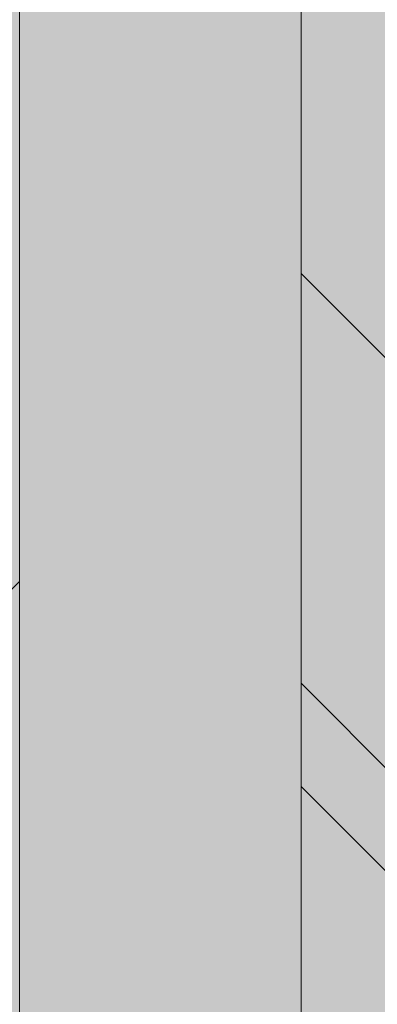
# Model space of a CAD drawing. Units: inches. Extents: x 844 to 2234, y 346 to 1084.
# Tile 78 of 93: x 1998.757 to 1999.568, y 706.514 to 708.742. Entities that reach past the tile are written whole.
import ezdxf

# ---------------------------------------------------------------- set-up
doc = ezdxf.new("R2010")
doc.units = ezdxf.units.IN
doc.header["$MEASUREMENT"] = 0
for name, color, linetype, lineweight in [('A-ANNO-DIMS', 2, 'Continuous', 18), ('furniture', 8, 'Continuous', 18), ('RA-AP-01$0$INT', 35, 'Continuous', 5)]:
    doc.layers.add(name, color=color, linetype=linetype, lineweight=lineweight)
doc.layers.add('RA-AP-01$0$FURN', color=3, linetype='Continuous')
doc.layers.add('RA-AP-01$0$WOOD', color=64, linetype='Continuous')
doc.styles.get("Standard").update_dxf_attribs({"font": 'arial.ttf'})
doc.dimstyles.get("Standard").update_dxf_attribs({"dimtxt": 6, "dimasz": 3, "dimexe": 0.18, "dimexo": 0.0625, "dimgap": 0.09, "dimtad": 0, "dimtih": 1, "dimtoh": 1, "dimdec": 1, "dimzin": 0, "dimdsep": 46, "dimlunit": 3, "dimtxsty": 'Standard', "dimblk": 'ARCHTICK', "dimcen": 0.09, "dimadec": 0, "dimazin": 0, "dimtfac": 1, "dimtdec": 1, "dimtofl": 0, "dimtmove": 0, "dimatfit": 3, "dimfxl": 1, "dimtolj": 1, "dimtzin": 0, "dimarcsym": 0})

# ---------------------------------------------------------------- blocks, each defined once
blk = doc.blocks.new('A$C18D01794')
at = {"layer": 'RA-AP-01$0$INT'}
h = blk.add_hatch(color=256, dxfattribs=at)
h.paths.add_polyline_path([(4.505206456958071, -7.585498806127123), (4.46934859260189, -7.549640941759413), (4.505206456958071, -7.513783077414768), (4.505206456958071, -7.381963272220687), (4.469348592616735, -7.346105407867824), (4.505206456958071, -7.310247543514964), (4.505206456958071, -7.178427738324996), (4.469348592586679, -7.142569873965138), (4.505206456952245, -7.106712009588038), (4.476922185709333, -7.106712009588038), (4.455206456960671, -7.128427738343681), (4.433490728198047, -7.106712009588038), (4.405206456946033, -7.106712009588036), (4.441064321339216, -7.142569873969684), (4.40520645695807, -7.178427738362358), (4.405206456958072, -7.310247543472698), (4.441064321364728, -7.346105407867826), (4.40520645695807, -7.381963272262947), (4.40520645695807, -7.513783077378263), (4.441064321354429, -7.549640941786153), (4.405206456958072, -7.585498806170974), (4.405206456958072, -7.717318611286652), (4.441064321333084, -7.753176475673194), (4.405206456958072, -7.789034340036673), (4.405206456958072, -8.006712009588039), (4.644348592588106, -8.006712009588039), (4.680206456964639, -7.970854145211967), (4.716064321341165, -8.006712009588039), (4.869348592586113, -8.006712009588039), (4.905206456964143, -7.970854145210465), (4.941064321342174, -8.006712009588039), (5.094348592587118, -8.006712009588037), (5.130206456963649, -7.970854145211967), (5.166064321340178, -8.006712009588039), (5.405206456958072, -8.006712009588039), (5.405206456958072, -7.789034340024526), (5.369348592595202, -7.753176475673196), (5.40520645695807, -7.717318611298797), (5.40520645695807, -7.585498806158829), (5.369348592573859, -7.549640941786151), (5.40520645695807, -7.51378307739041), (5.40520645695807, -7.381963272250803), (5.36934859256356, -7.346105407867824), (5.405206456958072, -7.310247543484846), (5.405206456958072, -7.178427738350217), (5.369348592589068, -7.142569873969682), (5.405206456982249, -7.106712009588038), (5.376922185730244, -7.106712009588038), (5.355206456967613, -7.128427738343679), (5.333490728218955, -7.10671200958804), (5.305206456976043, -7.106712009588042), (5.341064321341609, -7.142569873965136), (5.305206456958072, -7.178427738337141), (5.305206456958072, -7.310247543502816), (5.34106432131155, -7.346105407867824), (5.305206456958072, -7.381963272232832), (5.30520645695807, -7.513783077402624), (5.341064321326395, -7.549640941759413), (5.305206456958072, -7.585498806139263), (5.305206456958072, -7.717318611299605), (5.341064321347738, -7.753176475677737), (5.305206456958072, -7.78903434007894), (5.30520645695807, -7.906712009588039), (5.166064321336834, -7.906712009588039), (5.130206456963647, -7.942569873961684), (5.094348592590464, -7.906712009588039), (4.941064321338827, -7.906712009588041), (4.905206456964145, -7.942569873963183), (4.869348592589459, -7.906712009588039), (4.716064321337822, -7.906712009588041), (4.680206456964641, -7.942569873961684), (4.644348592591453, -7.906712009588039), (4.505206456958071, -7.906712009588039), (4.505206456958071, -7.789034340066795), (4.469348592580545, -7.753176475677738), (4.505206456958071, -7.717318611311748)])
h.paths.add_polyline_path([(4.485206456974132, -7.709034340046354), (4.45520645695909, -7.739034340051736), (4.425206456974128, -7.709034340057131), (4.425206456993394, -7.593783077384998), (4.45520645699153, -7.563783077396511), (4.485206456993396, -7.593783077408017)], flags=16)
h.paths.add_polyline_path([(4.455206456954537, -7.767318611299197), (4.485206456958242, -7.797318611312542), (4.48520645695951, -7.912569873958716), (4.45520645695415, -7.942569873954422), (4.425206456957888, -7.912569873967813), (4.425206456957888, -7.797318611286197)], flags=16)
h.paths.add_polyline_path([(4.455206456964794, -7.535498806149051), (4.42520645696469, -7.5054988061393), (4.425206456983954, -7.390247543486406), (4.455206456990734, -7.360247543489279), (4.485206456983953, -7.39024754349214), (4.485206456964687, -7.505498806158811)], flags=16)
h.paths.add_polyline_path([(4.499348592588947, -7.926712009585049), (4.636064321340932, -7.926712009585049), (4.666064321342317, -7.956712009586821), (4.636064321343707, -7.986712009585048), (4.499348592575121, -7.986712009585048), (4.469348592591685, -7.956712009591957)], flags=16)
h.paths.add_polyline_path([(4.425206456957888, -7.940854145195974), (4.471064321332215, -7.986712009585049), (4.425206456957888, -7.986712009585049)], flags=16)
h.paths.add_polyline_path([(4.455206456990734, -7.331963272246367), (4.425206456989053, -7.301963272254337), (4.425206456969784, -7.186712009596224), (4.455206456965226, -7.156712009591144), (4.485206456969787, -7.186712009586051), (4.485206456989053, -7.301963272238404)], flags=16)
h.paths.add_polyline_path([(4.72434859258714, -7.926712009586255), (4.861064321340141, -7.926712009586248), (4.891064321340324, -7.956712009586823), (4.861064321340513, -7.986712009586252), (4.724348592586768, -7.986712009586252), (4.694348592586956, -7.956712009586821)], flags=16)
h.paths.add_polyline_path([(4.919348592587961, -7.956712009586821), (4.949348592588145, -7.92671200958625), (5.08606432134115, -7.926712009586253), (5.116064321341327, -7.956712009586823), (5.086064321341519, -7.986712009586252), (4.949348592587774, -7.986712009586252)], flags=16)
h.paths.add_polyline_path([(5.144348592585967, -7.956712009586823), (5.174348592587358, -7.926712009585049), (5.311064321339338, -7.926712009585049), (5.3410643213366, -7.956712009591957), (5.311064321353163, -7.986712009585048), (5.174348592584576, -7.986712009585048)], flags=16)
h.paths.add_polyline_path([(5.32520645693489, -7.593783077408021), (5.355206456936755, -7.563783077396511), (5.385206456934894, -7.593783077384998), (5.38520645695416, -7.709034340057128), (5.355206456969194, -7.739034340051736), (5.325206456954153, -7.709034340046352)], flags=16)
h.paths.add_polyline_path([(5.325206456970042, -7.797318611312542), (5.355206456973747, -7.767318611299197), (5.385206456970398, -7.7973186112862), (5.385206456970398, -7.912569873967816), (5.355206456974136, -7.942569873954422), (5.325206456968778, -7.912569873958716)], flags=16)
h.paths.add_polyline_path([(5.325206456963599, -7.505498806158811), (5.325206456944333, -7.39024754349214), (5.355206456937552, -7.360247543489279), (5.385206456944332, -7.39024754348641), (5.385206456963596, -7.505498806139303), (5.355206456963492, -7.53549880614905)], flags=16)
h.paths.add_polyline_path([(5.32520645693923, -7.301963272238403), (5.3252064569585, -7.186712009586051), (5.355206456963062, -7.156712009591142), (5.3852064569585, -7.186712009596224), (5.385206456939234, -7.301963272254338), (5.355206456937552, -7.331963272246369)], flags=16)
h.paths.add_polyline_path([(5.339348592596071, -7.986712009585048), (5.385206456970398, -7.940854145195972), (5.385206456970396, -7.986712009585048)], flags=16)
h = blk.add_hatch(color=256, dxfattribs=at)
h.paths.add_polyline_path([(4.469348592586677, -7.142569873965136), (4.505206456958073, -7.178427738324996), (4.505206456958071, -7.106712009582215)])
h.paths.add_polyline_path([(4.455206456960671, -7.128427738343681), (4.476922185709333, -7.106712009588038), (4.433490728198045, -7.106712009588038)])
h.paths.add_polyline_path([(4.405206456958073, -7.178427738362358), (4.441064321339218, -7.142569873969684), (4.40520645695807, -7.106712009600073)])
h.paths.add_polyline_path([(4.425206456989053, -7.301963272254335), (4.455206456990736, -7.331963272246371), (4.485206456989055, -7.301963272238399), (4.48520645696979, -7.186712009586054), (4.455206456965227, -7.15671200959114), (4.425206456969784, -7.186712009596224)])
h.paths.add_polyline_path([(4.505206456958073, -7.381963272220689), (4.505206456958071, -7.310247543514961), (4.469348592616738, -7.346105407867826)])
h.paths.add_polyline_path([(4.425206456964688, -7.5054988061393), (4.455206456964794, -7.535498806149051), (4.485206456964689, -7.505498806158811), (4.485206456983951, -7.390247543492138), (4.455206456990736, -7.360247543489277), (4.425206456983956, -7.39024754348641)])
h.paths.add_polyline_path([(4.425206456974126, -7.709034340057128), (4.455206456959092, -7.739034340051736), (4.485206456974132, -7.709034340046356), (4.485206456993396, -7.593783077408017), (4.45520645699153, -7.563783077396511), (4.425206456993394, -7.593783077384999)])
h.paths.add_polyline_path([(4.46934859260189, -7.549640941759415), (4.505206456958071, -7.585498806127123), (4.505206456958073, -7.513783077414766)])
h.paths.add_polyline_path([(4.405206456958073, -7.585498806170972), (4.441064321354427, -7.549640941786151), (4.405206456958072, -7.513783077378263)])
h.paths.add_polyline_path([(4.405206456958072, -7.789034340036673), (4.441064321333084, -7.753176475673194), (4.405206456958072, -7.71731861128665)])
h.paths.add_polyline_path([(4.469348592580547, -7.75317647567774), (4.505206456958071, -7.789034340066795), (4.505206456958071, -7.717318611311744)])
h.paths.add_polyline_path([(4.425206456957888, -7.912569873967814), (4.45520645695415, -7.942569873954422), (4.485206456959507, -7.912569873958718), (4.48520645695824, -7.797318611312542), (4.455206456954537, -7.767318611299197), (4.425206456957888, -7.797318611286202)])
h.paths.add_polyline_path([(4.425206456957888, -7.986712009585049), (4.471064321332215, -7.986712009585049), (4.425206456957888, -7.940854145195972)])
h.paths.add_polyline_path([(4.499348592575121, -7.986712009585048), (4.636064321343707, -7.986712009585049), (4.666064321342317, -7.956712009586823), (4.636064321340932, -7.926712009585049), (4.499348592588945, -7.926712009585049), (4.469348592591685, -7.95671200959196)])
h.paths.add_polyline_path([(4.680206456964641, -7.942569873961684), (4.716064321337824, -7.906712009588039), (4.644348592591454, -7.906712009588039)])
h.paths.add_polyline_path([(4.644348592588108, -8.006712009588039), (4.716064321341167, -8.006712009588039), (4.680206456964637, -7.970854145211964)])
h.paths.add_polyline_path([(4.724348592586768, -7.98671200958625), (4.861064321340514, -7.986712009586252), (4.891064321340324, -7.956712009586819), (4.861064321340141, -7.92671200958625), (4.724348592587134, -7.926712009586255), (4.694348592586957, -7.956712009586821)])
h.paths.add_polyline_path([(4.905206456964143, -7.942569873963183), (4.941064321338827, -7.906712009588039), (4.869348592589457, -7.906712009588037)])
h.paths.add_polyline_path([(4.869348592586113, -8.006712009588039), (4.941064321342172, -8.006712009588037), (4.905206456964145, -7.970854145210463)])
h.paths.add_polyline_path([(4.949348592587774, -7.986712009586252), (5.086064321341521, -7.986712009586252), (5.116064321341329, -7.956712009586823), (5.08606432134115, -7.926712009586253), (4.949348592588145, -7.92671200958625), (4.919348592587961, -7.956712009586819)])
h.paths.add_polyline_path([(5.130206456963645, -7.942569873961684), (5.166064321336834, -7.906712009588039), (5.094348592590464, -7.906712009588039)])
h.paths.add_polyline_path([(5.094348592587119, -8.006712009588039), (5.166064321340178, -8.006712009588039), (5.130206456963651, -7.970854145211967)])
h.paths.add_polyline_path([(5.174348592584578, -7.986712009585048), (5.311064321353163, -7.986712009585048), (5.341064321336602, -7.956712009591958), (5.31106432133934, -7.926712009585049), (5.174348592587352, -7.926712009585049), (5.144348592585969, -7.956712009586823)])
h.paths.add_polyline_path([(5.325206456968778, -7.912569873958718), (5.355206456974136, -7.942569873954422), (5.385206456970396, -7.912569873967814), (5.385206456970396, -7.797318611286199), (5.355206456973747, -7.767318611299197), (5.325206456970044, -7.797318611312544)])
h.paths.add_polyline_path([(5.339348592596073, -7.986712009585048), (5.385206456970396, -7.986712009585049), (5.385206456970398, -7.94085414519597)])
h.paths.add_polyline_path([(5.325206456954155, -7.709034340046354), (5.355206456969194, -7.739034340051734), (5.38520645695416, -7.709034340057128), (5.385206456934896, -7.593783077384999), (5.355206456936758, -7.563783077396513), (5.325206456934888, -7.593783077408019)])
h.paths.add_polyline_path([(5.305206456958072, -7.789034340078938), (5.341064321347739, -7.753176475677738), (5.305206456958072, -7.717318611299605)])
h.paths.add_polyline_path([(5.369348592595204, -7.753176475673194), (5.40520645695807, -7.789034340024526), (5.405206456958072, -7.717318611298798)])
h.paths.add_polyline_path([(5.405206456958072, -7.585498806158831), (5.405206456958072, -7.513783077390407), (5.369348592573857, -7.549640941786151)])
h.paths.add_polyline_path([(5.305206456958072, -7.585498806139266), (5.341064321326393, -7.549640941759413), (5.305206456958072, -7.513783077402626)])
h.paths.add_polyline_path([(5.325206456963599, -7.50549880615881), (5.355206456963494, -7.535498806149055), (5.385206456963598, -7.505498806139302), (5.385206456944334, -7.390247543486411), (5.355206456937552, -7.360247543489279), (5.325206456944333, -7.39024754349214)])
h.paths.add_polyline_path([(5.305206456958072, -7.38196327223283), (5.341064321311551, -7.346105407867824), (5.305206456958072, -7.31024754350282)])
h.paths.add_polyline_path([(5.325206456939231, -7.301963272238404), (5.355206456937552, -7.331963272246369), (5.385206456939235, -7.301963272254335), (5.385206456958502, -7.186712009596224), (5.355206456963061, -7.156712009591142), (5.3252064569585, -7.186712009586051)])
h.paths.add_polyline_path([(5.404581768715993, -7.381338584008926, -0.001217816984214), (5.405206456958072, -7.381112009582329), (5.405206456958072, -7.310247543484846), (5.369348592563558, -7.346105407867826)])
h.paths.add_polyline_path([(5.36934859258907, -7.142569873969684), (5.40520645695807, -7.178427738350215), (5.405206456958072, -7.106712009612218)])
h.paths.add_polyline_path([(5.355206456967613, -7.128427738343683), (5.376922185730239, -7.106712009588038), (5.333490728218953, -7.10671200958804)])
h.paths.add_polyline_path([(5.30520645695807, -7.178427738337139), (5.341064321341609, -7.142569873965134), (5.305206456958074, -7.10671200957007)])
blk.add_hatch(color=256, dxfattribs=at).paths.add_polyline_path([(4.505206456958071, -7.906712009588039), (5.305206456958072, -7.906712009588039), (5.305206456958072, -7.106712009588038), (5.255206456951893, -7.106712009588036), (5.25520645694868, -7.856712009570104), (4.555206456959269, -7.856712009588616), (4.555206456956052, -7.106712009588038), (4.505206456958073, -7.106712009588038)])
h = blk.add_hatch(color=256, dxfattribs=at)
h.paths.add_polyline_path([(4.585917135068448, -7.856712009587804), (4.614201406330596, -7.856712009587056), (4.668846067270487, -7.802067348644738), (4.723490728212344, -7.856712009584164), (4.771774999457151, -7.856712009582887), (4.826419660396886, -7.80206734864072), (4.862780050090322, -7.838427738332541), (4.844495778842715, -7.856712009580965), (4.862780050090411, -7.856712009580482), (4.905206456960182, -7.814285602707865), (4.947632863832445, -7.856712009578238), (4.965917135079675, -7.856712009577755), (4.947632863831759, -7.838427738330656), (4.983993253523576, -7.802067348637219), (5.038637914464627, -7.856712009575829), (5.08692218571208, -7.856712009574554), (5.141566846649976, -7.802067348634224), (5.196211507589851, -7.856712009571666), (5.224495778822615, -7.856712009570916), (4.905206456953975, -7.537422687702283)])
h.paths.add_polyline_path([(4.895206456956031, -7.575706958950402), (4.895206456958921, -7.684996280828174), (4.840561796018589, -7.630351619890275)], flags=16)
h.paths.add_polyline_path([(4.915206456955638, -7.575706958949956), (4.969851117895509, -7.630351619887399), (4.915206456957609, -7.684996280827732)], flags=16)
h.paths.add_polyline_path([(4.826419660395175, -7.644493755514321), (4.881064321335613, -7.699138416452331), (4.771774999456703, -7.69913841645522)], flags=16)
h.paths.add_polyline_path([(4.983993253519558, -7.644493755510815), (5.038637914460456, -7.699138416449285), (4.929348592581548, -7.69913841645126)], flags=16)
h.paths.add_polyline_path([(4.881064321336025, -7.719138416452334), (4.826419660397532, -7.773783077393256), (4.771774999457062, -7.719138416455217)], flags=16)
h.paths.add_polyline_path([(4.929348592582019, -7.71913841645126), (5.038637914460982, -7.719138416449284), (4.983993253522945, -7.773783077389749)], flags=16)
h.paths.add_polyline_path([(4.895206456960191, -7.733280552075633), (4.895206456962115, -7.806001331460164), (4.876922185715016, -7.824285602708492), (4.840561796021581, -7.787925213016675)], flags=16)
h.paths.add_polyline_path([(4.915206456958487, -7.733280552075187), (4.969851117899527, -7.787925213013798), (4.933490728206909, -7.824285602708034), (4.9152064569598, -7.806001331461736)], flags=16)
h.paths.add_polyline_path([(4.757632863832376, -7.733280552079264), (4.812277524772842, -7.787925213017304), (4.757632863834348, -7.842569873958233)], flags=16)
h.paths.add_polyline_path([(4.737632863832376, -7.73328055207979), (4.737632863834348, -7.842569873958701), (4.682988202893906, -7.787925213020692)], flags=16)
h.paths.add_polyline_path([(5.05278005008503, -7.733280552072701), (5.052780050087917, -7.842569873951664), (4.998135389146995, -7.787925213013169)], flags=16)
h.paths.add_polyline_path([(5.072780050085024, -7.733280552072333), (5.127424711025931, -7.787925213010806), (5.072780050087916, -7.842569873951244)], flags=16)
h.paths.add_polyline_path([(4.935917135072783, -7.506712009583784), (5.255206456948811, -7.826001331459767), (5.255206456948932, -7.797717060211899), (5.200561796010279, -7.743072399273238), (5.255206456949403, -7.688427738334128), (5.25520645694961, -7.640143467086677), (5.200561796009787, -7.585498806146837), (5.236922185702417, -7.549138416454212), (5.255206456949919, -7.56742268770172), (5.255206456949998, -7.549138416454178), (5.212780050078687, -7.506712009583814), (5.25520645695036, -7.464285602712145), (5.255206456950438, -7.446001331464763), (5.236922185702424, -7.464285602712779), (5.200561796009796, -7.427925213020149), (5.255206456950753, -7.373280552079203), (5.25520645695096, -7.324996280834394), (5.200561796010322, -7.270351619893748), (5.255206456951428, -7.215706958952649), (5.255206456951547, -7.187422687705071)])
h.paths.add_polyline_path([(5.042988202883395, -7.42792521302065), (5.097632863823085, -7.373280552080975), (5.097632863822622, -7.482569873959883)], flags=16)
h.paths.add_polyline_path([(5.028846067259663, -7.442067348644384), (5.083490728198774, -7.496712009583504), (4.974201406321001, -7.496712009583035)], flags=16)
h.paths.add_polyline_path([(5.117632863823087, -7.37328055208089), (5.172277524762331, -7.42792521302015), (5.11763286382262, -7.482569873959851)], flags=16)
h.paths.add_polyline_path([(5.08349072819877, -7.516712009582191), (5.028846067259652, -7.571356670521302), (4.974201406320998, -7.516712009582638)], flags=16)
h.paths.add_polyline_path([(5.131774999446817, -7.35913841645716), (5.186419660386065, -7.413783077396415), (5.241064321325782, -7.359138416456712)], flags=17)
h.paths.add_polyline_path([(5.131774999446228, -7.496712009583703), (5.186419660386065, -7.442067348643883), (5.222780050079488, -7.478427738337313), (5.204495778832781, -7.496712009584014)], flags=16)
h.paths.add_polyline_path([(5.097632863822613, -7.530854145205813), (5.097632863823061, -7.640143467084723), (5.042988202883383, -7.585498806145032)], flags=16)
h.paths.add_polyline_path([(5.131774999446899, -7.339138416457162), (5.241064321325809, -7.339138416456712), (5.186419660386591, -7.284493755517479)], flags=17)
h.paths.add_polyline_path([(5.131774999446226, -7.516712009581999), (5.204495778830767, -7.516712009581702), (5.22278005007868, -7.534996280829206), (5.186419660386049, -7.571356670521828)], flags=16)
h.paths.add_polyline_path([(5.11763286382262, -7.530854145205852), (5.17227752476232, -7.585498806145562), (5.117632863823064, -7.64014346708481)], flags=16)
h.paths.add_polyline_path([(5.186419660386069, -7.599640941770585), (5.241064321325754, -7.654285602710281), (5.131774999446791, -7.654285602709814)], flags=16)
h.paths.add_polyline_path([(5.131774999446872, -7.674285602709813), (5.24106432132578, -7.674285602710282), (5.186419660386554, -7.728930263649504)], flags=16)
h.paths.add_polyline_path([(5.255206456951811, -7.126001331467467), (5.255206456951895, -7.106712009588038), (4.555206456956052, -7.106712009588038), (4.555206456956136, -7.12600133146746), (4.905206456953973, -7.476001331465289)])
h.paths.add_polyline_path([(4.983993253513404, -7.368930263651977), (4.92934859257295, -7.314285602713969), (5.03863791445186, -7.314285602711063)], flags=16)
h.paths.add_polyline_path([(4.969851117889988, -7.383072399276016), (4.915206456952556, -7.437717060215906), (4.915206456949648, -7.328427738338133)], flags=16)
h.paths.add_polyline_path([(4.929348592572535, -7.294285602713971), (4.983993253511019, -7.239640941773039), (5.038637914451496, -7.294285602711065)], flags=16)
h.paths.add_polyline_path([(5.052780050074912, -7.280143467087016), (4.998135389134438, -7.225498806148989), (5.052780050072919, -7.170854145208052)], flags=16)
h.paths.add_polyline_path([(5.07278005007491, -7.280143467086489), (5.072780050072918, -7.170854145207579), (5.127424711013374, -7.225498806145578)], flags=16)
h.paths.add_polyline_path([(4.89520645695295, -7.437717060216355), (4.840561796013067, -7.383072399278919), (4.895206456950961, -7.328427738338582)], flags=16)
h.paths.add_polyline_path([(4.915206456948365, -7.280143467090674), (4.915206456946434, -7.207422687704125), (4.933490728192729, -7.18913841645701), (4.969851117886972, -7.225498806149623)], flags=16)
h.paths.add_polyline_path([(4.881064321327021, -7.314285602715054), (4.82641966038902, -7.368930263655506), (4.771774999448108, -7.314285602717047)], flags=16)
h.paths.add_polyline_path([(4.895206456950073, -7.280143467091125), (4.840561796009022, -7.225498806152518), (4.876922185700835, -7.18913841645908), (4.895206456948749, -7.207422687706589)], flags=16)
h.paths.add_polyline_path([(4.983993253510392, -7.211356670525576), (4.947632863816944, -7.174996280833758), (4.965917135064043, -7.156712009585847), (5.038637914448995, -7.156712009584522)], flags=16)
h.paths.add_polyline_path([(4.881064321326543, -7.294285602715056), (4.771774999447578, -7.294285602717046), (4.826419660385607, -7.239640941776569)], flags=16)
h.paths.add_polyline_path([(4.905206456946447, -7.19913841645844), (4.862780050074785, -7.156712009587725), (4.947632863816685, -7.156712009586302)], flags=16)
h.paths.add_polyline_path([(5.14156684663679, -7.211356670521528), (5.086922185696452, -7.156712009583639), (5.196211507574223, -7.156712009581651)], flags=16)
h.paths.add_polyline_path([(4.8264196603837, -7.211356670529104), (4.771774999442643, -7.156712009590501), (4.8444957788276, -7.156712009588568), (4.862780050075511, -7.17499628083566)], flags=16)
h.paths.add_polyline_path([(4.812277524760289, -7.225498806153156), (4.757632863822258, -7.28014346709363), (4.757632863819352, -7.170854145214669)], flags=16)
h.paths.add_polyline_path([(4.73763286382226, -7.280143467093997), (4.682988202881349, -7.22549880615554), (4.737632863819352, -7.170854145215086)], flags=16)
h.paths.add_polyline_path([(4.723490728195188, -7.156712009591787), (4.668846067257299, -7.211356670532127), (4.614201406317417, -7.156712009594693)], flags=16)
h.paths.add_polyline_path([(4.597632863829262, -7.506712009583814), (4.555206456957951, -7.54913841645418), (4.555206456958029, -7.56742268770172), (4.573490728205535, -7.549138416454212), (4.609851117898167, -7.585498806146839), (4.555206456958338, -7.640143467086675), (4.555206456958546, -7.688427738334125), (4.60985111789767, -7.743072399273238), (4.555206456959015, -7.797717060211899), (4.555206456959138, -7.826001331459767), (4.874495778835167, -7.506712009583786), (4.5552064569564, -7.187422687705062), (4.555206456956523, -7.215706958952644), (4.609851117897629, -7.270351619893746), (4.555206456956988, -7.324996280834396), (4.555206456957198, -7.373280552079195), (4.609851117898153, -7.427925213020147), (4.573490728205528, -7.464285602712779), (4.555206456957507, -7.446001331464756), (4.555206456957585, -7.464285602712143)])
h.paths.add_polyline_path([(4.712780050085332, -7.482569873959882), (4.712780050084863, -7.373280552080972), (4.767424711024555, -7.42792521302065)], flags=16)
h.paths.add_polyline_path([(4.726922185709173, -7.496712009583504), (4.781566846648288, -7.442067348644384), (4.836211507586949, -7.496712009583033)], flags=16)
h.paths.add_polyline_path([(4.692780050085327, -7.482569873959851), (4.638135389145619, -7.427925213020149), (4.692780050084865, -7.373280552080892)], flags=16)
h.paths.add_polyline_path([(4.726922185709182, -7.516712009582191), (4.836211507586949, -7.51671200958264), (4.7815668466483, -7.571356670521304)], flags=16)
h.paths.add_polyline_path([(4.678637914461726, -7.496712009583706), (4.605917135075169, -7.496712009584014), (4.587632863828464, -7.478427738337311), (4.623993253521887, -7.442067348643881)], flags=16)
h.paths.add_polyline_path([(4.712780050085336, -7.530854145205816), (4.767424711024568, -7.585498806145034), (4.71278005008489, -7.640143467084724)], flags=16)
h.paths.add_polyline_path([(4.678637914461726, -7.516712009582001), (4.623993253521899, -7.571356670521829), (4.587632863829271, -7.534996280829206), (4.605917135077185, -7.5167120095817)], flags=16)
h.paths.add_polyline_path([(4.692780050085336, -7.530854145205848), (4.692780050084889, -7.64014346708481), (4.638135389145632, -7.585498806145562)], flags=16)
h.paths.add_polyline_path([(4.623993253521885, -7.413783077396415), (4.678637914461131, -7.359138416457161), (4.56934859258217, -7.359138416456712)], flags=17)
h.paths.add_polyline_path([(4.623993253521901, -7.599640941770568), (4.678637914461158, -7.654285602709814), (4.569348592582195, -7.654285602710281)], flags=16)
h.paths.add_polyline_path([(4.678637914461051, -7.339138416457162), (4.623993253521361, -7.284493755517479), (4.569348592582143, -7.339138416456712)], flags=17)
h.paths.add_polyline_path([(4.678637914461076, -7.674285602709813), (4.623993253521399, -7.728930263649504), (4.569348592582167, -7.674285602710281)], flags=16)
h = blk.add_hatch(color=256, dxfattribs=at)
h.paths.add_polyline_path([(5.028846067259997, -7.571356670520955), (4.974201406321342, -7.516712009582294), (5.083490728199115, -7.516712009581846)])
h.paths.add_polyline_path([(4.974201406321344, -7.496712009582688), (5.028846067260004, -7.442067348644037), (5.083490728199117, -7.496712009583157)])
h.paths.add_polyline_path([(5.042988202883738, -7.427925213020309), (5.097632863823428, -7.373280552080627), (5.097632863822963, -7.482569873959537)])
h.paths.add_polyline_path([(5.117632863822961, -7.482569873959509), (5.117632863823428, -7.373280552080546), (5.172277524762674, -7.427925213019804)])
h.paths.add_polyline_path([(5.131774999446572, -7.496712009583358), (5.186419660386406, -7.442067348643536), (5.222780050079831, -7.478427738336961), (5.204495778833122, -7.496712009583667)])
h.paths.add_polyline_path([(5.236922185702764, -7.464285602712433), (5.200561796010139, -7.427925213019802), (5.255206456949971, -7.373280552079975), (5.255206456950271, -7.446001331464927)])
h.paths.add_polyline_path([(5.186419660386412, -7.41378307739607), (5.131774999447164, -7.359138416456815), (5.241064321326123, -7.359138416456366)])
h.paths.add_polyline_path([(5.131774999447238, -7.339138416456815), (5.186419660386934, -7.284493755517132), (5.241064321326153, -7.339138416456368)])
h.paths.add_polyline_path([(5.200561796010663, -7.270351619893402), (5.255206456949324, -7.215706958954747), (5.255206456949777, -7.324996280832518)])
h.paths.add_polyline_path([(5.21278005007903, -7.50671200958347), (5.255206456950223, -7.464285602712278), (5.255206456950696, -7.549138416454185)])
h.paths.add_polyline_path([(5.13177499944657, -7.516712009581652), (5.204495778831106, -7.516712009581354), (5.222780050079024, -7.534996280828858), (5.186419660386397, -7.571356670521485)])
h.paths.add_polyline_path([(5.117632863823405, -7.640143467084465), (5.117632863822955, -7.530854145205498), (5.172277524762665, -7.585498806145217)])
h.paths.add_polyline_path([(5.042988202883727, -7.585498806144689), (5.097632863822957, -7.530854145205474), (5.097632863823407, -7.64014346708438)])
h.paths.add_polyline_path([(5.131774999447135, -7.654285602709467), (5.186419660386394, -7.599640941770219), (5.241064321326097, -7.654285602709933)])
h.paths.add_polyline_path([(5.200561796010128, -7.585498806146492), (5.236922185702758, -7.549138416453866), (5.255206456950264, -7.567422687701371), (5.255206456949948, -7.640143467086325)])
h.paths.add_polyline_path([(5.186419660386895, -7.728930263649157), (5.131774999447213, -7.674285602709467), (5.241064321326127, -7.674285602709934)])
h.paths.add_polyline_path([(5.200561796010624, -7.743072399272893), (5.255206456949745, -7.688427738333778), (5.255206456949276, -7.797717060211553)])
for p, q in [((5.255206456951895, -7.106712009588038), (5.255206456948681, -7.856712009570104)), ((5.25520645694988, -7.464285602712626), (5.255206456950353, -7.549138416454534)), ((5.212780050078687, -7.506712009583814), (5.255206456950353, -7.549138416454534)), ((5.255206456949919, -7.56742268770172), (5.236922185702415, -7.549138416454212)), ((5.305206456939818, -7.58549880615752), (5.341064321310754, -7.549640941775056)), ((5.255206456949918, -7.56742268770172), (5.255206456949605, -7.640143467086671)), ((5.255206456949605, -7.640143467086671), (5.200561796009783, -7.585498806146837))]:
    blk.add_line(p, q, dxfattribs=at)
blk.add_lwpolyline([(5.305206456958072, -7.106712009588038), (5.305206456958072, -7.906712009588039), (4.505206456958071, -7.906712009588039), (4.505206456958071, -7.106712009588038)], dxfattribs=at)
blk = doc.blocks.new('A$C32926AE1')
at = {"layer": 'RA-AP-01$0$WOOD'}
h = blk.add_hatch(color=256, dxfattribs=at)
h.dxf.hatch_style = 1
h.paths.add_polyline_path([(5.157430609644524, 4.573483066760929, -0.1009492694046607), (5.155401577623758, 4.593365984175333, -0.1842662638101597), (5.172249623284174, 4.638795604568598, 0.2056608120311276), (5.179560981299304, 4.661316324430096, 0.3614336704623542), (5.134352340494423, 4.706524965234944, 0.2056608120311297), (5.111831620632933, 4.699213607219793, -0.1842662638101113), (5.066402000239693, 4.682365561559342, -0.1055311479399994), (5.045656153913092, 4.68467289944697, 0.1567636581983829), (4.763886414745334, 4.684672899446966, -0.1055311479399895), (4.743140568418733, 4.68236556155934, -0.1842662638100833), (4.6977109480255, 4.69921360721979, 0.2056608120302612), (4.675190228164109, 4.706524965234949, 0.3614336704708441), (4.629981587358889, 4.66131632442871, 0.2056608120245944), (4.637292945374126, 4.638795604567974, -0.1842662638101024), (4.654140991034615, 4.59336598417475, -0.1009492694055169), (4.652111959013835, 4.573483066760181, 0.021410119221476), (4.629748025606143, 4.156712009541676, 0.0214101192214795), (4.652111959013809, 3.739940952323101, -0.1009492694059586), (4.654140991034615, 3.720058034908448, -0.1842662638100975), (4.637292945374126, 3.674628414515226, 0.2056608120245705), (4.629981587358889, 3.652107694654492, 0.3614336704708879), (4.675190228164113, 3.606899053848249, 0.2056608120302384), (4.697710948025501, 3.614210411863408, -0.1842662638100995), (4.743140568418738, 3.63105845752386, -0.1055311479402541), (4.763886414745388, 3.628751119636215, 0.1567636581983776), (5.045656153913137, 3.628751119636244, -0.1055311479397538), (5.066402000239692, 3.631058457523857, -0.1842662638101067), (5.111831620632931, 3.614210411863407, 0.2056608120310924), (5.134352340494417, 3.606899053848256, 0.3614336704624001), (5.179560981299307, 3.652107694653103, 0.2056608120311314), (5.172249623284175, 3.6746284145146, -0.1842662638101402), (5.155401577623758, 3.72005803490786, -0.1009492694051366), (5.15743060964455, 3.739940952322354, 0.0214101192215073), (5.179794543052287, 4.156712009541468, 0.0214101192215252)])
h.paths.add_polyline_path([(4.639748609479751, 4.156712009541513, 0.0213537860821624), (4.661970494867118, 3.741887061152232, -0.094075836301374), (4.664143710413708, 3.7196126951003, -0.1824818158568985), (4.644813765429836, 3.668037719127816, 0.2056608120245319), (4.639939526753007, 3.653023905887301, 0.3614336704710246), (4.676106439397173, 3.616856993242342, 0.2056608120302234), (4.691120252638095, 3.621731231919122, -0.1824818158602558), (4.742695228611606, 3.641061176902986, -0.1029891339458722), (4.766991894714349, 3.638256818950944, 0.156709409989566), (5.042550673941472, 3.638256818950105, -0.102989133958497), (5.066847340047078, 3.641061176902949, -0.1824818158594995), (5.118422316020358, 3.621731231919103, 0.2056608120311416), (5.133436129261316, 3.616856993242346, 0.3614336704621468), (5.169603041905217, 3.653023905886178, 0.2056608120310986), (5.164728803228477, 3.668037719127177, -0.1824818158565612), (5.145398858244737, 3.719612695099578, -0.0940758363009313), (5.147572073791232, 3.741887061151398, 0.0213537860822023), (5.169793959178681, 4.156712009541451, 0.0213537860822226), (5.147572073791203, 4.571536957931898, -0.0940758363005034), (5.145398858244737, 4.59381132398362, -0.1824818158565587), (5.164728803228476, 4.645386299956021, 0.2056608120311045), (5.169603041905216, 4.66040011319702, 0.3614336704621845), (5.133436129261313, 4.696567025840856, 0.2056608120310773), (5.118422316020359, 4.691692787164098, -0.182481815859508), (5.066847340047078, 4.67236284218025, -0.1029891339584606), (5.04255067394148, 4.675167200133092, 0.156709409989566), (4.766991894714357, 4.675167200132257, -0.1029891339458842), (4.742695228611611, 4.672362842180213, -0.1824818158602725), (4.691120252638095, 4.691692787164077, 0.2056608120302152), (4.676106439397174, 4.696567025840858, 0.3614336704710363), (4.639939526753005, 4.660400113195899, 0.2056608120245495), (4.644813765429837, 4.645386299955384, -0.1824818158568934), (4.664143710413708, 4.593811323982902, -0.0940758363009187), (4.661970494867149, 4.571536957931074, 0.021353786082177)], flags=16)
h.paths.add_polyline_path([(5.129794543052235, 4.432167055276933, -0.0141661062790638), (5.130152669293814, 4.156927903047693, -0.0141661062790647), (5.129794543052234, 3.881688750818433, -0.0785247771143638), (5.10979738006795, 3.755143611847103, 0.0945969212073497), (5.105408519571111, 3.717898134952927, 0.1043170707844957), (5.116074640131521, 3.670385395016088, 0.1043170707864965), (5.068561900193738, 3.681051515576561, 0.09459692119553), (5.031316423304057, 3.676662655080835, -0.1580239521427272), (4.778226145355827, 3.676662655080367, 0.0945969211986668), (4.740980668464973, 3.681051515576592, 0.1043170707882822), (4.693467928526415, 3.670385395015844, 0.1043170707867916), (4.704134049087309, 3.717898134953662, 0.0945969211972894), (4.69974518859162, 3.755143611844042, -0.0785247771163196), (4.679748025606343, 3.881688750818406, -0.0141661062790663), (4.679389899364763, 4.156927903047693, -0.0141661062790672), (4.679748025606343, 4.432167055276998, -0.0785247771163064), (4.699745188591625, 4.55871219425134, 0.094596921197333), (4.704134049087308, 4.595957671141738, 0.1043170707867205), (4.693467928526416, 4.643470411079523, 0.1043170707882628), (4.740980668464965, 4.632804290518776, 0.0945969211988114), (4.778226145355874, 4.637193151015016, -0.158023952142669), (5.031316423304015, 4.637193151014546, 0.0945969211956361), (5.068561900193736, 4.632804290518806, 0.1043170707864979), (5.11607464013152, 4.643470411079278, 0.1043170707844617), (5.105408519571112, 4.595957671142455, 0.0945969212074597), (5.109797380067959, 4.558712194248236, -0.0785247771143467)], flags=0)
h.paths.add_polyline_path([(5.119794532311105, 4.432259799204851, -0.0142000800617244), (5.120156169157484, 4.156927903047701, -0.0142000800617277), (5.119794532311105, 3.881596006890482, -0.0784894509520253), (5.100273383573699, 3.758192358677797, 0.0940138827242913), (5.095413455884425, 3.717477693979438, 0.0606271852308753), (5.099615656341024, 3.686844378806616, 0.0606271852322524), (5.068982341167493, 3.691046579263239, 0.0940138827010453), (5.028267676478798, 3.686186651576848, -0.1580706864508061), (4.781274892180912, 3.686186651576435, 0.0940138827026903), (4.740560227491556, 3.691046579263279, 0.0606271852339895), (4.709926912317155, 3.686844378806508, 0.0606271852329405), (4.714129112773991, 3.717477693980356, 0.094013882701304), (4.709269185087677, 3.758192358669163, -0.0784894509577193), (4.689748036347473, 3.881596006890469, -0.014200080061729), (4.689386399501094, 4.156927903047709, -0.0142000800617217), (4.689748036347473, 4.432259799204808, -0.078489450957724), (4.709269185087651, 4.555663447426125, 0.0940138827014585), (4.714129112773992, 4.596378112114996, 0.0606271852329731), (4.709926912317154, 4.62701142728886, 0.0606271852340196), (4.74056022749157, 4.622809226832087, 0.0940138827024997), (4.781274892180847, 4.627669154518912, -0.1580706864508359), (5.028267676478777, 4.627669154518526, 0.0940138827010946), (5.068982341167492, 4.622809226832129, 0.060627185232254), (5.099615656341024, 4.627011427288751, 0.0606271852308727), (5.095413455884425, 4.59637811211593, 0.0940138827241088), (5.100273383573675, 4.555663447417647, -0.0784894509520978)], flags=0)
h.paths.add_polyline_path([(5.06978912287499, 4.430218106756144, -0.014241683694547), (5.070173729147532, 4.156927903047672, -0.0142416836945458), (5.06978912287499, 3.883637699339223, -0.0800609523125196), (5.052662118612511, 3.773463122773442, 0.0526421978001116), (5.04590916754064, 3.740550867606997, 0.0526421977992423), (5.012996912374707, 3.73379791653534, -0.1583028414718258), (4.796545656286308, 3.73379791653451, 0.0526421978034211), (4.763633401117837, 3.740550867607021, 0.0526421978018622), (4.756880450045755, 3.773463122774558, -0.0800609523117106), (4.739753445783639, 3.883637699339268, -0.0142416836945435), (4.739368839511098, 4.156927903047671, -0.0142416836945477), (4.739753445783639, 4.430218106756155, -0.0800609523116345), (4.75688045004574, 4.540392683320762, 0.052642197801941), (4.763633401117837, 4.573304938488346, 0.0526421978035071), (4.796545656286361, 4.580057889560873, -0.1583028414717561), (5.012996912374669, 4.580057889560039, 0.0526421977993048), (5.04590916754064, 4.57330493848837, 0.0526421978002057), (5.052662118612529, 4.540392683321868, -0.080060952312477)], flags=0)
h.paths.add_polyline_path([(5.049789715110557, 4.43038092723357, -0.0143097550741839), (5.05018085590259, 4.156927903047715, -0.0143097550741854), (5.049789715110558, 3.883474878861827, -0.0800685599149176), (5.03362098255317, 3.779581877367999, 0.0306258898956367), (5.028241146483733, 3.758218888663947, 0.0306258898977031), (5.006878157778253, 3.75283905259408, -0.1583983521624096), (4.802664410878162, 3.752839052594731, 0.0306258898946014), (4.781301422174808, 3.758218888663924, 0.0306258898967912), (4.775921586105202, 3.779581877368794, -0.080068559914251), (4.759752853548071, 3.883474878861786, -0.0143097550741854), (4.759361712756037, 4.156927903047671, -0.0143097550741854), (4.759752853548071, 4.430380927233557, -0.0800685599142479), (4.775921586105193, 4.534273928726546, 0.0306258898968306), (4.781301422174808, 4.555636917431444, 0.0306258898945754), (4.802664410878143, 4.561016753500631, -0.1583983521624168), (5.006878157778244, 4.561016753501291, 0.0306258898977177), (5.028241146483733, 4.555636917431421, 0.0306258898958182), (5.03362098255321, 4.534273928727244, -0.080068559914796)], flags=0)
h.paths.add_polyline_path([(4.999766070382627, 4.428171244713864, -0.0143443147609634), (5.000198441819402, 4.156927903047689, -0.0143443147609612), (4.999766070382627, 3.885684561381556, -0.0784641635803329), (4.987356730658798, 3.799103304488872, -0.1506053783831347), (4.822185837999821, 3.79910330448882, -0.0784641635803318), (4.809776498276007, 3.885684561381509, -0.014344314760963), (4.809344126839227, 4.156927903047677, -0.0143443147609645), (4.809776498276007, 4.428171244713873, -0.0784641635803192), (4.822185837999822, 4.514752501606549, -0.1506053783831338), (4.987356730658798, 4.514752501606494, -0.078464163580285)], flags=0)
h.paths.add_polyline_path([(4.979755254238824, 4.42764379880488, -0.0143772539198268), (4.980205517789977, 4.156927903047693, -0.0143772539198275), (4.979755254238824, 3.886212007290489, -0.0689242507424422), (4.971183264704897, 3.815276770442801, -0.1296645318904179), (4.838359303953726, 3.815276770442746, -0.0689242507424186), (4.829787314419809, 3.886212007290419, -0.0143772539198292), (4.829337050868653, 4.156927903047653, -0.0143772539198325), (4.829787314419809, 4.427643798804946, -0.0689242507424211), (4.838359303953725, 4.498579035652621, -0.1296645318904187), (4.971183264704897, 4.498579035652565, -0.0689242507424401)], flags=0)
blk.add_arc((0.304323780376417, 4.104079819130551), 4.875754844654793, 0.6185013483537143, 5.524589681839913, dxfattribs=at)
blk = doc.blocks.new('A$C5D2F253E')
at = {"layer": 'RA-AP-01$0$FURN', "xscale": -0.7999999999883585, "yscale": 0.7999999999883585, "zscale": 0.8, "rotation": 90}
blk.add_blockref('A$C18D01794', (-5.687757199772477, 4.75791982714071), dxfattribs=at)
at = {"layer": 'RA-AP-01$0$WOOD', "rotation": 270}
blk.add_blockref('A$C32926AE1', (-4.161339601644158, 5.73852594588169), dxfattribs=at)
blk = doc.blocks.new('_ArchTick')
at = {"color": 0, "linetype": 'ByBlock', "const_width": 0.15}
blk.add_lwpolyline([(-0.5, -0.5), (0.5, 0.5)], dxfattribs=at)
blk = doc.blocks.new('*D121')
at = {"layer": 'A-ANNO-DIMS', "color": 0, "lineweight": -2, "transparency": 16777216}
for p, q in [((2030.271987351997, 734.262611118704), (2040.245275089302, 734.262611118704)), ((2040.065275089302, 734.262611118704), (2040.065275089302, 704.6043509484256)), ((2040.065275089302, 668.557359536674), (2040.065275089302, 698.2156197069523)), ((2030.271987351997, 668.557359536674), (2040.245275089302, 668.557359536674))]:
    blk.add_line(p, q, dxfattribs=at)
at = {"layer": 'Defpoints', "color": 0, "transparency": 16777216}
for p in [(2030.209487351997, 734.262611118704), (2040.065275089302, 734.262611118704), (2030.209487351997, 668.557359536674)]:
    blk.add_point(p, dxfattribs=at)
at = {"layer": 'A-ANNO-DIMS', "color": 0, "lineweight": -2, "transparency": 16777216, "xscale": 3, "yscale": 3, "zscale": 3}
for p, rotation in [((2040.065275089302, 734.262611118704), 90), ((2040.065275089302, 668.557359536674), 270)]:
    blk.add_blockref('_ArchTick', p, dxfattribs=dict(at, rotation=rotation))
at = {"layer": 'A-ANNO-DIMS', "color": 0, "transparency": 16777216, "insert": (2040.065275089302, 701.4099853276883), "char_height": 6, "attachment_point": 5}
blk.add_mtext('\\A1;LOUNGE SET 5\'-5 1/2" TYP.', dxfattribs=at)

msp = doc.modelspace()

# ---------------------------------------------------------------- block references
at = {"layer": 'furniture', "xscale": -15.94108302203742, "yscale": 15.94108302203742, "zscale": 15.94108302203742, "rotation": 270}
msp.add_blockref('A$C5D2F253E', (1990.567271852805, 701.4028671565849), dxfattribs=at)

# ---------------------------------------------------------------- dimensions: what is measured, and where the dimension line sits
at = {"layer": 'A-ANNO-DIMS'}
dim = msp.add_linear_dim(base=(2040.065275089302, 734.262611118704), p1=(2030.209487351996, 668.5573595366737), p2=(2030.209487351996, 734.2626111187037), angle=90, text='LOUNGE SET <> TYP.', dimstyle='Standard', override={"dimdec": 1, "dimlfac": 1, "dimrnd": 0, "dimzin": 1, "dimdsep": 46, "dimlunit": 4, "dimfrac": 2}, dxfattribs=at)
dim.commit()
dim.dimension.update_dxf_attribs({"geometry": '*D121', "text_midpoint": (2040.065275089302, 701.4099853276883)})

doc.saveas('drawing.dxf')
